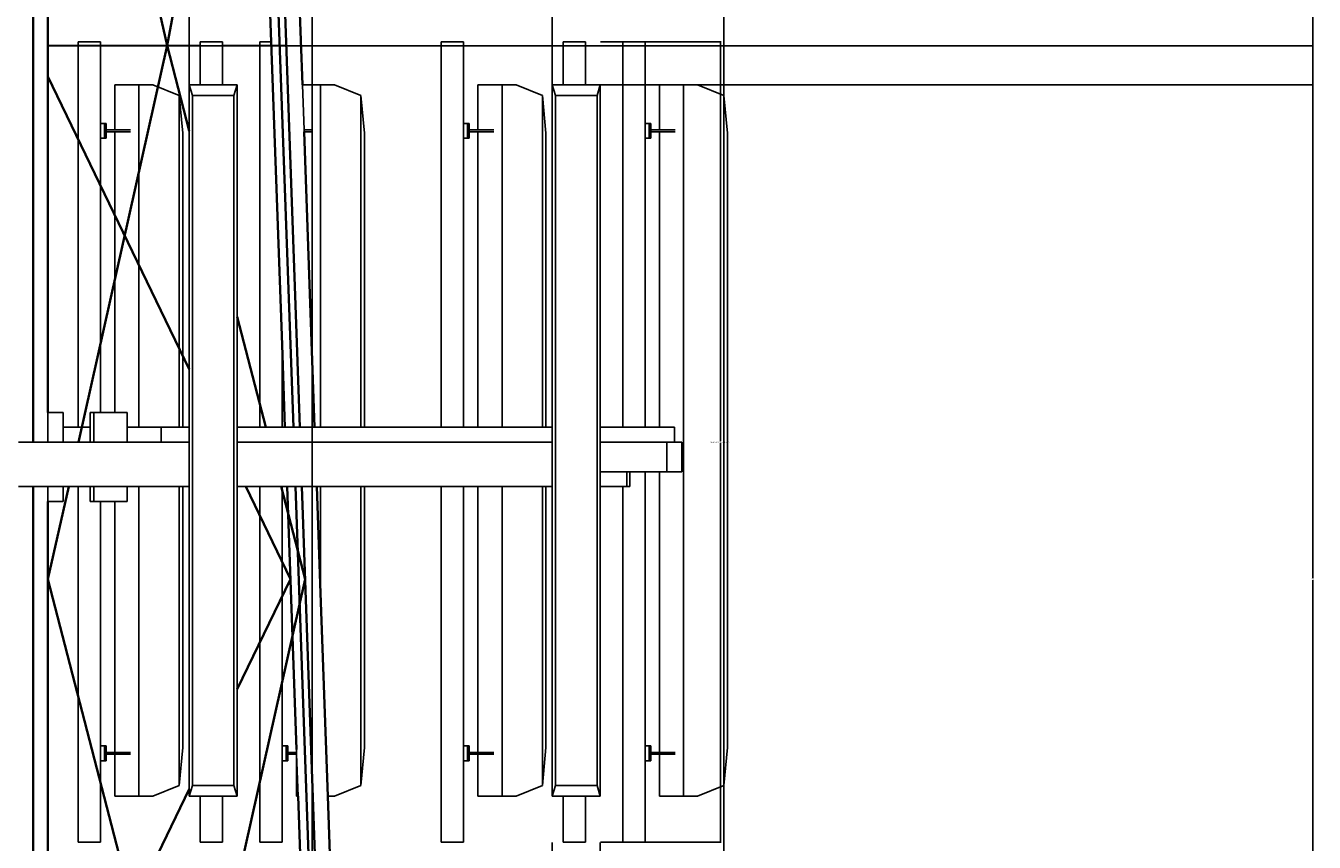
# Model space of a CAD drawing. Units: inches. Extents: x 3780 to 4301, y 1637 to 4224.
# Tile 3 of 8: x 4040 to 4301, y 3092 to 3257. Entities that reach past the tile are written whole.
import ezdxf

# ---------------------------------------------------------------- set-up
doc = ezdxf.new("R2010")
doc.units = ezdxf.units.IN
for name, color, linetype, lineweight in [('A-ANNO-DIMS', 2, 'Continuous', 18), ('E-COMM-ANTN', 4, 'Continuous', 25), ('S-TOWR', 7, 'Continuous', 35)]:
    doc.layers.add(name, color=color, linetype=linetype, lineweight=lineweight)
doc.styles.get("Standard").update_dxf_attribs({"font": 'arial.ttf'})
doc.dimstyles.get("Standard").update_dxf_attribs({"dimtxt": 0.18, "dimasz": 0.18, "dimexe": 0.18, "dimexo": 0.0625, "dimgap": 0.09, "dimtad": 0, "dimtih": 1, "dimtoh": 1, "dimdec": 4, "dimzin": 0, "dimdsep": 46, "dimtxsty": 'Standard', "dimcen": 0.09, "dimadec": 0, "dimazin": 0, "dimtfac": 1, "dimtdec": 4, "dimtofl": 0, "dimtmove": 0, "dimatfit": 3, "dimfxl": 1, "dimtolj": 1, "dimtzin": 0, "dimarcsym": 0})

# ---------------------------------------------------------------- blocks, each defined once
blk = doc.blocks.new('ANT-PANEL')
for p, q in [((3905.38, 3835.91), (3900.05, 3833.75)), ((3905.38, 3835.91), (3908.22, 3835.91)), ((3908.22, 3691.91), (3908.22, 3835.91)), ((3900.05, 3833.75), (3899.34, 3826.07)), ((3900.05, 3694.07), (3900.05, 3833.75)), ((3899.34, 3701.75), (3899.34, 3826.07)), ((3900.05, 3694.07), (3899.34, 3701.75)), ((3905.38, 3691.91), (3900.05, 3694.07)), ((3905.38, 3691.91), (3908.22, 3691.91))]:
    blk.add_line(p, q)
blk = doc.blocks.new('ANT-PANEL-MOUNT-B')
for p, q in [((4148.97, 3835.91), (4148.97, 3844.56)), ((4153.47, 3844.56), (4148.97, 3844.56)), ((4153.47, 3835.91), (4153.47, 3844.56)), ((4146.73, 3835.91), (4147.4, 3833.75)), ((4146.73, 3835.91), (4148.97, 3835.91)), ((4146.73, 3766.56), (4146.73, 3835.91)), ((4148.97, 3835.91), (4153.47, 3835.91)), ((4153.47, 3835.91), (4156.48, 3835.91)), ((4156.48, 3835.91), (4155.82, 3833.75)), ((4156.48, 3766.56), (4156.48, 3835.91)), ((4147.4, 3833.75), (4155.82, 3833.75)), ((4147.4, 3694.07), (4147.4, 3833.75)), ((4155.82, 3694.07), (4155.82, 3833.75)), ((4146.73, 3763.56), (4146.73, 3766.56)), ((4156.48, 3763.56), (4156.48, 3766.56)), ((4146.73, 3754.56), (4146.73, 3763.56)), ((4156.48, 3757.56), (4156.48, 3763.56)), ((4156.48, 3754.56), (4156.48, 3757.56)), ((4146.73, 3691.91), (4146.73, 3754.56)), ((4156.48, 3691.91), (4156.48, 3754.56)), ((4146.73, 3691.91), (4147.4, 3694.07)), ((4147.4, 3694.07), (4155.82, 3694.07)), ((4156.48, 3691.91), (4155.82, 3694.07)), ((4146.73, 3691.91), (4148.97, 3691.91)), ((4148.97, 3682.56), (4148.97, 3691.91)), ((4148.97, 3691.91), (4153.47, 3691.91)), ((4153.47, 3682.56), (4153.47, 3691.91)), ((4153.47, 3691.91), (4156.48, 3691.91)), ((4148.97, 3682.56), (4153.47, 3682.56))]:
    blk.add_line(p, q)
blk = doc.blocks.new('*D9')
at = {"layer": 'A-ANNO-DIMS', "color": 0, "lineweight": -2, "transparency": 16777216}
for p, q in [((4156.54, 3254.21), (4180.96, 3254.21)), ((4180.78, 3254.03), (4180.78, 3173.4)), ((4180.78, 3092.39), (4180.78, 3173.03)), ((4156.54, 3092.21), (4180.96, 3092.21))]:
    blk.add_line(p, q, dxfattribs=at)
at = {"layer": 'A-ANNO-DIMS', "color": 0, "transparency": 16777216}
for points in [[(4180.75, 3254.03), (4180.81, 3254.03), (4180.78, 3254.21)], [(4180.75, 3092.39), (4180.81, 3092.39), (4180.78, 3092.21)]]:
    blk.add_solid(points, dxfattribs=at)
at = {"layer": 'Defpoints', "color": 0, "transparency": 16777216}
for p in [(4156.48, 3254.21), (4180.78, 3254.21), (4156.48, 3092.21)]:
    blk.add_point(p, dxfattribs=at)
at = {"layer": 'A-ANNO-DIMS', "color": 0, "transparency": 16777216, "insert": (4180.78, 3173.21), "char_height": 0.18, "attachment_point": 5}
blk.add_mtext('\\A1;PANEL ANTENNA MOUNT B 162 TYP.', dxfattribs=at)
blk = doc.blocks.new('*D10')
at = {"layer": 'A-ANNO-DIMS', "color": 0, "lineweight": -2, "transparency": 16777216}
for p, q in [((4146.73, 3092.15), (4146.73, 3067.73)), ((4156.48, 3092.15), (4156.48, 3067.73)), ((4146.91, 3067.91), (4151.09, 3067.91)), ((4156.3, 3067.91), (4152.13, 3067.91))]:
    blk.add_line(p, q, dxfattribs=at)
at = {"layer": 'A-ANNO-DIMS', "color": 0, "transparency": 16777216}
for points in [[(4146.91, 3067.94), (4146.91, 3067.88), (4146.73, 3067.91)], [(4156.3, 3067.94), (4156.3, 3067.88), (4156.48, 3067.91)]]:
    blk.add_solid(points, dxfattribs=at)
at = {"layer": 'Defpoints', "color": 0, "transparency": 16777216}
for p in [(4146.73, 3092.21), (4156.48, 3092.21), (4156.48, 3067.91)]:
    blk.add_point(p, dxfattribs=at)
at = {"layer": 'A-ANNO-DIMS', "color": 0, "transparency": 16777216, "insert": (4151.61, 3067.91), "char_height": 0.18, "attachment_point": 5}
blk.add_mtext('\\A1;10 TYP.', dxfattribs=at)
blk = doc.blocks.new('*D19')
at = {"layer": 'A-ANNO-DIMS', "color": 0, "lineweight": -2, "transparency": 16777216}
for p, q in [((4044.72, 3253.46), (4300.89, 3253.46)), ((4300.71, 3253.28), (4300.71, 3145.65)), ((4300.71, 3037.64), (4300.71, 3145.28)), ((4044.72, 3037.46), (4300.89, 3037.46))]:
    blk.add_line(p, q, dxfattribs=at)
at = {"layer": 'A-ANNO-DIMS', "color": 0, "transparency": 16777216}
for points in [[(4300.68, 3253.28), (4300.74, 3253.28), (4300.71, 3253.46)], [(4300.68, 3037.64), (4300.74, 3037.64), (4300.71, 3037.46)]]:
    blk.add_solid(points, dxfattribs=at)
at = {"layer": 'Defpoints', "color": 0, "transparency": 16777216}
for p in [(4044.66, 3253.46), (4300.71, 3253.46), (4044.66, 3037.46)]:
    blk.add_point(p, dxfattribs=at)
at = {"layer": 'A-ANNO-DIMS', "color": 0, "transparency": 16777216, "insert": (4300.71, 3145.46), "char_height": 0.18, "attachment_point": 5}
blk.add_mtext('\\A1;216', dxfattribs=at)
blk = doc.blocks.new('*D20')
at = {"layer": 'A-ANNO-DIMS', "color": 0, "lineweight": -2, "transparency": 16777216}
for p, q in [((4044.72, 3469.46), (4300.89, 3469.46)), ((4300.71, 3469.28), (4300.71, 3361.65)), ((4300.71, 3253.64), (4300.71, 3361.28)), ((4044.72, 3253.46), (4300.89, 3253.46))]:
    blk.add_line(p, q, dxfattribs=at)
at = {"layer": 'A-ANNO-DIMS', "color": 0, "transparency": 16777216}
for points in [[(4300.68, 3469.28), (4300.74, 3469.28), (4300.71, 3469.46)], [(4300.68, 3253.64), (4300.74, 3253.64), (4300.71, 3253.46)]]:
    blk.add_solid(points, dxfattribs=at)
at = {"layer": 'Defpoints', "color": 0, "transparency": 16777216}
for p in [(4044.66, 3469.46), (4300.71, 3469.46), (4044.66, 3253.46)]:
    blk.add_point(p, dxfattribs=at)
at = {"layer": 'A-ANNO-DIMS', "color": 0, "transparency": 16777216, "insert": (4300.71, 3361.46), "char_height": 0.18, "attachment_point": 5}
blk.add_mtext('\\A1;216', dxfattribs=at)
blk = doc.blocks.new('*D22')
at = {"layer": 'A-ANNO-DIMS', "color": 0, "lineweight": -2, "transparency": 16777216}
for p, q in [((3900.05, 3694.01), (3900.05, 1636.57)), ((4181.5, 3694.01), (4181.5, 1636.57)), ((3900.23, 1636.75), (4040.31, 1636.75)), ((4181.32, 1636.75), (4041.24, 1636.75))]:
    blk.add_line(p, q, dxfattribs=at)
at = {"layer": 'A-ANNO-DIMS', "color": 0, "transparency": 16777216}
for points in [[(3900.23, 1636.78), (3900.23, 1636.72), (3900.05, 1636.75)], [(4181.32, 1636.78), (4181.32, 1636.72), (4181.5, 1636.75)]]:
    blk.add_solid(points, dxfattribs=at)
at = {"layer": 'Defpoints', "color": 0, "transparency": 16777216}
for p in [(3900.05, 3694.07), (4181.5, 3694.07), (4181.5, 1636.75)]:
    blk.add_point(p, dxfattribs=at)
at = {"layer": 'A-ANNO-DIMS', "color": 0, "transparency": 16777216, "insert": (4040.77, 1636.75), "char_height": 0.18, "attachment_point": 5}
blk.add_mtext('\\A1;281.45', dxfattribs=at)
blk = doc.blocks.new('*D27')
at = {"layer": 'A-ANNO-DIMS', "color": 0, "lineweight": -2, "transparency": 16777216}
for p, q in [((4048.31, 3488.69), (3780.66, 3488.69)), ((3780.84, 3488.51), (3780.84, 3295.31)), ((3780.84, 3101.74), (3780.84, 3294.94)), ((3926.17, 3101.56), (3780.66, 3101.56))]:
    blk.add_line(p, q, dxfattribs=at)
at = {"layer": 'A-ANNO-DIMS', "color": 0, "transparency": 16777216}
for points in [[(3780.81, 3488.51), (3780.87, 3488.51), (3780.84, 3488.69)], [(3780.81, 3101.74), (3780.87, 3101.74), (3780.84, 3101.56)]]:
    blk.add_solid(points, dxfattribs=at)
at = {"layer": 'Defpoints', "color": 0, "transparency": 16777216}
for p in [(3780.84, 3488.69), (4048.37, 3488.69), (3926.23, 3101.56)]:
    blk.add_point(p, dxfattribs=at)
at = {"layer": 'A-ANNO-DIMS', "color": 0, "transparency": 16777216, "insert": (3780.84, 3295.13), "char_height": 0.18, "attachment_point": 5}
blk.add_mtext('\\A1;387.1', dxfattribs=at)
blk = doc.blocks.new('*D42')
at = {"layer": 'A-ANNO-DIMS', "color": 0, "lineweight": -2, "transparency": 16777216}
for p, q in [((3997.15, 3538.4), (3997.15, 1636.57)), ((4098.15, 3539.64), (4098.15, 1636.57)), ((3997.33, 1636.75), (4047.38, 1636.75)), ((4097.97, 1636.75), (4047.91, 1636.75))]:
    blk.add_line(p, q, dxfattribs=at)
at = {"layer": 'A-ANNO-DIMS', "color": 0, "transparency": 16777216}
for points in [[(3997.33, 1636.78), (3997.33, 1636.72), (3997.15, 1636.75)], [(4097.97, 1636.78), (4097.97, 1636.72), (4098.15, 1636.75)]]:
    blk.add_solid(points, dxfattribs=at)
at = {"layer": 'Defpoints', "color": 0, "transparency": 16777216}
for p in [(3997.15, 3538.47), (4098.15, 3539.7), (4098.15, 1636.75)]:
    blk.add_point(p, dxfattribs=at)
at = {"layer": 'A-ANNO-DIMS', "color": 0, "transparency": 16777216, "insert": (4047.65, 1636.75), "char_height": 0.18, "attachment_point": 5}
blk.add_mtext('\\A1;101', dxfattribs=at)
blk = doc.blocks.new('*D49')
at = {"layer": 'A-ANNO-DIMS', "color": 0, "lineweight": -2, "transparency": 16777216}
for p, q in [((3999.73, 3245.63), (3999.73, 4223.96)), ((3999.91, 4223.78), (4036.16, 4223.78)), ((4073.05, 4223.78), (4036.81, 4223.78)), ((4073.23, 3245.63), (4073.23, 4223.96))]:
    blk.add_line(p, q, dxfattribs=at)
at = {"layer": 'A-ANNO-DIMS', "color": 0, "transparency": 16777216}
for points in [[(3999.91, 4223.81), (3999.91, 4223.75), (3999.73, 4223.78)], [(4073.05, 4223.81), (4073.05, 4223.75), (4073.23, 4223.78)]]:
    blk.add_solid(points, dxfattribs=at)
at = {"layer": 'Defpoints', "color": 0, "transparency": 16777216}
for p in [(4073.23, 4223.78), (3999.73, 3245.56), (4073.23, 3245.56)]:
    blk.add_point(p, dxfattribs=at)
at = {"layer": 'A-ANNO-DIMS', "color": 0, "transparency": 16777216, "insert": (4036.48, 4223.78), "char_height": 0.18, "attachment_point": 5}
blk.add_mtext('\\A1;73.5', dxfattribs=at)
blk = doc.blocks.new('*D50')
at = {"layer": 'A-ANNO-DIMS', "color": 0, "lineweight": -2, "transparency": 16777216}
for p, q in [((4073.23, 3245.63), (4073.23, 4223.96)), ((4073.41, 4223.78), (4109.66, 4223.78)), ((4146.55, 4223.78), (4110.31, 4223.78)), ((4146.73, 3245.63), (4146.73, 4223.96))]:
    blk.add_line(p, q, dxfattribs=at)
at = {"layer": 'A-ANNO-DIMS', "color": 0, "transparency": 16777216}
for points in [[(4073.41, 4223.81), (4073.41, 4223.75), (4073.23, 4223.78)], [(4146.55, 4223.81), (4146.55, 4223.75), (4146.73, 4223.78)]]:
    blk.add_solid(points, dxfattribs=at)
at = {"layer": 'Defpoints', "color": 0, "transparency": 16777216}
for p in [(4146.73, 4223.78), (4073.23, 3245.56), (4146.73, 3245.56)]:
    blk.add_point(p, dxfattribs=at)
at = {"layer": 'A-ANNO-DIMS', "color": 0, "transparency": 16777216, "insert": (4109.98, 4223.78), "char_height": 0.18, "attachment_point": 5}
blk.add_mtext('\\A1;73.5', dxfattribs=at)
blk = doc.blocks.new('*D60')
at = {"layer": 'A-ANNO-DIMS', "color": 0, "lineweight": -2, "transparency": 16777216}
for p, q in [((4170.32, 3280.03), (4300.89, 3280.03)), ((4300.71, 3279.85), (4300.71, 3262.98)), ((4300.71, 3245.74), (4300.71, 3262.62)), ((4156.54, 3245.56), (4300.89, 3245.56))]:
    blk.add_line(p, q, dxfattribs=at)
at = {"layer": 'A-ANNO-DIMS', "color": 0, "transparency": 16777216}
for points in [[(4300.68, 3279.85), (4300.74, 3279.85), (4300.71, 3280.03)], [(4300.68, 3245.74), (4300.74, 3245.74), (4300.71, 3245.56)]]:
    blk.add_solid(points, dxfattribs=at)
at = {"layer": 'Defpoints', "color": 0, "transparency": 16777216}
for p in [(4170.26, 3280.03), (4300.71, 3280.03), (4156.48, 3245.56)]:
    blk.add_point(p, dxfattribs=at)
at = {"layer": 'A-ANNO-DIMS', "color": 0, "transparency": 16777216, "insert": (4300.71, 3262.8), "char_height": 0.18, "attachment_point": 5}
blk.add_mtext('\\A1;34.47', dxfattribs=at)

msp = doc.modelspace()

# ---------------------------------------------------------------- linework, layer by layer
at = {"layer": 'E-COMM-ANTN'}
for p, q in [((4044.6622, 3253.4644), (4068.7741, 3253.4644)), ((4075.4676, 3253.4644), (4044.6622, 3253.4644)), ((4050.7911, 3176.2144), (4050.7911, 3254.2144)), ((4050.7911, 3254.2144), (4055.2911, 3254.2144)), ((4055.2911, 3237.7144), (4055.2911, 3254.2144)), ((4068.7741, 3253.4644), (4075.4676, 3253.4644)), ((4075.4676, 3245.5639), (4075.4676, 3254.2144)), ((4075.4676, 3254.2144), (4079.9676, 3254.2144)), ((4079.9676, 3245.5639), (4079.9676, 3254.2144)), ((4089.886, 3253.4644), (4079.9676, 3253.4644)), ((4079.9676, 3253.4644), (4092.886, 3253.4644)), ((4087.5411, 3176.2144), (4087.5411, 3254.2144)), ((4087.5411, 3254.2144), (4089.8594, 3254.2144)), ((4124.2911, 3176.2144), (4124.2911, 3254.2144)), ((4124.2911, 3254.2144), (4128.7911, 3254.2144)), ((4128.7911, 3237.7144), (4128.7911, 3254.2144)), ((4161.0411, 3176.2144), (4161.0411, 3254.2144)), ((4165.5411, 3254.2144), (4161.0411, 3254.2144)), ((4165.5411, 3237.7144), (4165.5411, 3254.2144)), ((4058.2034, 3236.4019), (4058.2034, 3245.5639)), ((4058.2034, 3245.5639), (4063.0784, 3245.5639)), ((4063.0784, 3245.5639), (4065.9127, 3245.5639)), ((4063.0784, 3176.2144), (4063.0784, 3245.5639)), ((4065.9127, 3245.5639), (4071.248, 3243.4039)), ((4073.2315, 3245.5639), (4073.8979, 3243.4039)), ((4073.2315, 3245.5639), (4075.4676, 3245.5639)), ((4073.2315, 3176.2144), (4073.2315, 3245.5639)), ((4075.4676, 3245.5639), (4079.9676, 3245.5639)), ((4079.9676, 3245.5639), (4082.9815, 3245.5639)), ((4082.9815, 3245.5639), (4082.3151, 3243.4039)), ((4082.9815, 3176.2144), (4082.9815, 3245.5639)), ((4096.4929, 3236.4019), (4096.167, 3245.5639)), ((4096.167, 3245.5639), (4099.8284, 3245.5639)), ((4099.8284, 3176.2144), (4099.8284, 3245.5639)), ((4099.8284, 3245.5639), (4102.6627, 3245.5639)), ((4102.6627, 3245.5639), (4107.998, 3243.4039)), ((4131.7034, 3236.4019), (4131.7034, 3245.5639)), ((4131.7034, 3245.5639), (4136.5784, 3245.5639)), ((4136.5784, 3176.2144), (4136.5784, 3245.5639)), ((4136.5784, 3245.5639), (4139.4127, 3245.5639)), ((4139.4127, 3245.5639), (4144.748, 3243.4039)), ((4168.4534, 3236.4019), (4168.4534, 3245.5639)), ((4168.4534, 3245.5639), (4173.3284, 3245.5639)), ((4071.248, 3176.2144), (4071.248, 3243.4039)), ((4071.248, 3243.4039), (4071.9591, 3235.7215)), ((4073.8979, 3103.7239), (4073.8979, 3243.4039)), ((4073.8979, 3243.4039), (4082.3151, 3243.4039)), ((4082.3151, 3103.7239), (4082.3151, 3243.4039)), ((4107.998, 3243.4039), (4108.7091, 3235.7215)), ((4107.998, 3176.2144), (4107.998, 3243.4039)), ((4144.748, 3243.4039), (4145.4591, 3235.7215)), ((4144.748, 3176.2144), (4144.748, 3243.4039)), ((4055.2911, 3237.7144), (4056.1147, 3237.7144)), ((4055.2911, 3234.7144), (4055.2911, 3237.7144)), ((4056.1147, 3237.7144), (4056.4394, 3237.7144)), ((4056.1147, 3234.7144), (4056.1147, 3237.7144)), ((4056.4394, 3237.7144), (4056.4394, 3236.4019)), ((4128.7911, 3237.7144), (4129.6147, 3237.7144)), ((4128.7911, 3234.7144), (4128.7911, 3237.7144)), ((4129.6147, 3237.7144), (4129.9394, 3237.7144)), ((4129.6147, 3234.7144), (4129.6147, 3237.7144)), ((4129.9394, 3237.7144), (4129.9394, 3236.4019)), ((4165.5411, 3237.7144), (4166.3647, 3237.7144)), ((4165.5411, 3234.7144), (4165.5411, 3237.7144)), ((4166.3647, 3234.7144), (4166.3647, 3237.7144)), ((4166.3647, 3237.7144), (4166.6894, 3237.7144)), ((4166.6894, 3237.7144), (4166.6894, 3236.4019)), ((4055.2911, 3234.7144), (4056.1147, 3234.7144)), ((4055.2911, 3179.2144), (4055.2911, 3234.7144)), ((4056.1147, 3234.7144), (4056.4394, 3234.7144)), ((4058.2034, 3236.4019), (4056.4394, 3236.4019)), ((4056.4394, 3236.4019), (4056.4394, 3236.0269)), ((4056.4394, 3236.0269), (4058.2034, 3236.0269)), ((4056.4394, 3236.0269), (4056.4394, 3234.7144)), ((4058.2034, 3236.4019), (4061.3979, 3236.4019)), ((4058.2034, 3179.2144), (4058.2034, 3236.0269)), ((4058.2034, 3236.0269), (4061.3979, 3236.0269)), ((4071.9591, 3176.2144), (4071.9591, 3235.7215)), ((4096.5062, 3236.0269), (4096.4929, 3236.4019)), ((4096.4929, 3236.4019), (4098.1479, 3236.4019)), ((4096.5062, 3236.0269), (4098.1479, 3236.0269)), ((4108.7091, 3176.2144), (4108.7091, 3235.7215)), ((4128.7911, 3234.7144), (4129.6147, 3234.7144)), ((4128.7911, 3176.2144), (4128.7911, 3234.7144)), ((4129.6147, 3234.7144), (4129.9394, 3234.7144)), ((4131.7034, 3236.4019), (4129.9394, 3236.4019)), ((4129.9394, 3236.4019), (4129.9394, 3236.0269)), ((4129.9394, 3236.0269), (4131.7034, 3236.0269)), ((4129.9394, 3236.0269), (4129.9394, 3234.7144)), ((4131.7034, 3236.4019), (4134.8979, 3236.4019)), ((4131.7034, 3176.2144), (4131.7034, 3236.0269)), ((4131.7034, 3236.0269), (4134.8979, 3236.0269)), ((4145.4591, 3176.2144), (4145.4591, 3235.7215)), ((4165.5411, 3234.7144), (4166.3647, 3234.7144)), ((4165.5411, 3176.2144), (4165.5411, 3234.7144)), ((4166.3647, 3234.7144), (4166.6894, 3234.7144)), ((4166.6894, 3236.4019), (4168.4534, 3236.4019)), ((4166.6894, 3236.4019), (4166.6894, 3236.0269)), ((4166.6894, 3236.0269), (4166.6894, 3234.7144)), ((4166.6894, 3236.0269), (4168.4534, 3236.0269)), ((4168.4534, 3236.4019), (4171.6479, 3236.4019)), ((4168.4534, 3176.2144), (4168.4534, 3236.0269)), ((4168.4534, 3236.0269), (4171.6479, 3236.0269)), ((4092.0411, 3176.2144), (4092.0411, 3192.8708)), ((4047.7176, 3179.2144), (4044.6622, 3179.2144)), ((4044.6622, 3173.2144), (4044.6622, 3179.2144)), ((4047.7176, 3176.2144), (4047.7176, 3179.2144)), ((4053.9472, 3179.2144), (4053.181, 3179.2144)), ((4053.181, 3176.2144), (4053.181, 3179.2144)), ((4053.9472, 3173.2144), (4053.9472, 3179.2144)), ((4053.9472, 3179.2144), (4055.2911, 3179.2144)), ((4055.2911, 3179.2144), (4058.2034, 3179.2144)), ((4060.6972, 3179.2144), (4058.2034, 3179.2144)), ((4060.6972, 3179.2144), (4060.6972, 3176.2144)), ((4047.7176, 3173.2144), (4047.7176, 3176.2144)), ((4047.7176, 3176.2144), (4050.7911, 3176.2144)), ((4050.7911, 3176.2144), (4053.181, 3176.2144)), ((4053.181, 3173.2144), (4053.181, 3176.2144)), ((4060.6972, 3176.2144), (4060.6972, 3173.2144)), ((4060.6972, 3176.2144), (4063.0784, 3176.2144)), ((4063.0784, 3176.2144), (4067.5445, 3176.2144)), ((4067.5445, 3173.2144), (4067.5445, 3176.2144)), ((4071.248, 3176.2144), (4067.5445, 3176.2144)), ((4071.9591, 3176.2144), (4071.248, 3176.2144)), ((4073.2315, 3176.2144), (4071.9591, 3176.2144)), ((4073.2315, 3173.2144), (4073.2315, 3176.2144)), ((4087.5411, 3176.2144), (4082.9815, 3176.2144)), ((4082.9815, 3173.2144), (4082.9815, 3176.2144)), ((4092.0411, 3176.2144), (4087.5411, 3176.2144)), ((4092.6335, 3176.2144), (4092.0411, 3176.2144)), ((4094.3345, 3176.2144), (4092.6335, 3176.2144)), ((4095.6335, 3176.2144), (4094.3345, 3176.2144)), ((4098.6335, 3176.2144), (4095.6335, 3176.2144)), ((4099.8284, 3176.2144), (4098.6335, 3176.2144)), ((4107.998, 3176.2144), (4099.8284, 3176.2144)), ((4108.7091, 3176.2144), (4107.998, 3176.2144)), ((4124.2911, 3176.2144), (4108.7091, 3176.2144)), ((4128.7911, 3176.2144), (4124.2911, 3176.2144)), ((4131.7034, 3176.2144), (4128.7911, 3176.2144)), ((4136.5784, 3176.2144), (4131.7034, 3176.2144)), ((4144.748, 3176.2144), (4136.5784, 3176.2144)), ((4145.4591, 3176.2144), (4144.748, 3176.2144)), ((4146.7315, 3176.2144), (4145.4591, 3176.2144)), ((4161.0411, 3176.2144), (4156.4815, 3176.2144)), ((4165.5411, 3176.2144), (4161.0411, 3176.2144)), ((4168.4534, 3176.2144), (4165.5411, 3176.2144)), ((4171.4676, 3176.2144), (4168.4534, 3176.2144)), ((4171.4676, 3173.2144), (4171.4676, 3176.2144)), ((4041.6622, 3173.2144), (4038.6622, 3173.2144)), ((4044.6622, 3173.2144), (4041.6622, 3173.2144)), ((4047.7176, 3173.2144), (4044.6622, 3173.2144)), ((4053.181, 3173.2144), (4047.7176, 3173.2144)), ((4053.9472, 3173.2144), (4053.181, 3173.2144)), ((4053.9472, 3173.2144), (4060.6972, 3173.2144)), ((4067.5445, 3173.2144), (4060.6972, 3173.2144)), ((4073.2315, 3173.2144), (4067.5445, 3173.2144)), ((4073.2315, 3164.2144), (4073.2315, 3173.2144)), ((4146.7315, 3173.2144), (4082.9815, 3173.2144)), ((4082.9815, 3164.2144), (4082.9815, 3173.2144)), ((4169.976, 3173.2144), (4156.4815, 3173.2144)), ((4169.976, 3167.2144), (4169.976, 3173.2144)), ((4169.976, 3173.2144), (4171.4676, 3173.2144)), ((4172.9591, 3173.2144), (4171.4676, 3173.2144)), ((4172.9591, 3173.2144), (4172.9591, 3167.2144)), ((4161.818, 3167.2144), (4156.4815, 3167.2144)), ((4161.818, 3164.2144), (4161.818, 3167.2144)), ((4162.4676, 3167.2144), (4161.818, 3167.2144)), ((4162.4676, 3164.2144), (4162.4676, 3167.2144)), ((4165.5411, 3167.2144), (4162.4676, 3167.2144)), ((4165.5411, 3111.7144), (4165.5411, 3167.2144)), ((4168.4534, 3167.2144), (4165.5411, 3167.2144)), ((4168.4534, 3110.4019), (4168.4534, 3167.2144)), ((4169.976, 3167.2144), (4168.4534, 3167.2144)), ((4172.9591, 3167.2144), (4169.976, 3167.2144)), ((4038.6622, 3164.2144), (4041.6622, 3164.2144)), ((4041.6622, 3164.2144), (4044.6622, 3164.2144)), ((4044.6622, 3161.2144), (4044.6622, 3164.2144)), ((4044.6622, 3164.2144), (4047.7176, 3164.2144)), ((4047.7176, 3161.2144), (4047.7176, 3164.2144)), ((4047.7176, 3164.2144), (4050.7911, 3164.2144)), ((4050.7911, 3092.2144), (4050.7911, 3164.2144)), ((4050.7911, 3164.2144), (4053.181, 3164.2144)), ((4053.181, 3161.2144), (4053.181, 3164.2144)), ((4053.181, 3164.2144), (4053.9472, 3164.2144)), ((4053.9472, 3161.2144), (4053.9472, 3164.2144)), ((4053.9472, 3164.2144), (4060.6972, 3164.2144)), ((4060.6972, 3164.2144), (4060.6972, 3161.2144)), ((4060.6972, 3164.2144), (4063.0784, 3164.2144)), ((4063.0784, 3101.5639), (4063.0784, 3164.2144)), ((4063.0784, 3164.2144), (4071.248, 3164.2144)), ((4071.248, 3103.7239), (4071.248, 3164.2144)), ((4071.248, 3164.2144), (4071.9591, 3164.2144)), ((4071.9591, 3111.4063), (4071.9591, 3164.2144)), ((4071.9591, 3164.2144), (4073.2315, 3164.2144)), ((4073.2315, 3101.5639), (4073.2315, 3164.2144)), ((4082.9815, 3164.2144), (4087.5411, 3164.2144)), ((4082.9815, 3101.5639), (4082.9815, 3164.2144)), ((4087.5411, 3092.2144), (4087.5411, 3164.2144)), ((4087.5411, 3164.2144), (4092.0411, 3164.2144)), ((4092.0411, 3111.7144), (4092.0411, 3164.2144)), ((4092.0411, 3164.2144), (4093.0603, 3164.2144)), ((4093.0603, 3164.2144), (4094.7613, 3164.2144)), ((4094.7613, 3164.2144), (4096.0603, 3164.2144)), ((4096.0603, 3164.2144), (4099.0603, 3164.2144)), ((4099.0603, 3164.2144), (4099.8284, 3164.2144)), ((4099.8284, 3142.6188), (4099.8284, 3164.2144)), ((4099.8284, 3164.2144), (4107.998, 3164.2144)), ((4107.998, 3103.7239), (4107.998, 3164.2144)), ((4107.998, 3164.2144), (4108.7091, 3164.2144)), ((4108.7091, 3111.4063), (4108.7091, 3164.2144)), ((4108.7091, 3164.2144), (4124.2911, 3164.2144)), ((4124.2911, 3092.2144), (4124.2911, 3164.2144)), ((4124.2911, 3164.2144), (4128.7911, 3164.2144)), ((4128.7911, 3111.7144), (4128.7911, 3164.2144)), ((4128.7911, 3164.2144), (4131.7034, 3164.2144)), ((4131.7034, 3110.4019), (4131.7034, 3164.2144)), ((4131.7034, 3164.2144), (4136.5784, 3164.2144)), ((4136.5784, 3101.5639), (4136.5784, 3164.2144)), ((4136.5784, 3164.2144), (4144.748, 3164.2144)), ((4144.748, 3103.7239), (4144.748, 3164.2144)), ((4144.748, 3164.2144), (4145.4591, 3164.2144)), ((4145.4591, 3111.4063), (4145.4591, 3164.2144)), ((4145.4591, 3164.2144), (4146.7315, 3164.2144)), ((4156.4815, 3164.2144), (4161.0411, 3164.2144)), ((4161.0411, 3092.2144), (4161.0411, 3164.2144)), ((4161.818, 3164.2144), (4161.0411, 3164.2144)), ((4162.4676, 3164.2144), (4161.818, 3164.2144)), ((4044.6622, 3161.2144), (4047.7176, 3161.2144)), ((4053.9472, 3161.2144), (4053.181, 3161.2144)), ((4055.2911, 3161.2144), (4053.9472, 3161.2144)), ((4058.2034, 3161.2144), (4055.2911, 3161.2144)), ((4055.2911, 3111.7144), (4055.2911, 3161.2144)), ((4058.2034, 3110.4019), (4058.2034, 3161.2144)), ((4060.6972, 3161.2144), (4058.2034, 3161.2144)), ((4055.2911, 3111.7144), (4056.1147, 3111.7144)), ((4055.2911, 3108.7144), (4055.2911, 3111.7144)), ((4056.1147, 3111.7144), (4056.4394, 3111.7144)), ((4056.1147, 3108.7144), (4056.1147, 3111.7144)), ((4056.4394, 3111.7144), (4056.4394, 3110.4019)), ((4058.2034, 3110.4019), (4056.4394, 3110.4019)), ((4056.4394, 3110.4019), (4056.4394, 3110.0269)), ((4056.4394, 3110.0269), (4058.2034, 3110.0269)), ((4056.4394, 3110.0269), (4056.4394, 3108.7144)), ((4058.2034, 3110.4019), (4061.3979, 3110.4019)), ((4058.2034, 3101.5639), (4058.2034, 3110.0269)), ((4058.2034, 3110.0269), (4061.3979, 3110.0269)), ((4071.248, 3103.7239), (4071.9591, 3111.4063)), ((4092.0411, 3111.7144), (4092.8647, 3111.7144)), ((4092.0411, 3108.7144), (4092.0411, 3111.7144)), ((4092.8647, 3108.7144), (4092.8647, 3111.7144)), ((4092.8647, 3111.7144), (4093.1894, 3111.7144)), ((4093.1894, 3111.7144), (4093.1894, 3110.4019)), ((4094.9534, 3110.4019), (4093.1894, 3110.4019)), ((4093.1894, 3110.4019), (4093.1894, 3110.0269)), ((4093.1894, 3110.0269), (4093.1894, 3108.7144)), ((4093.1894, 3110.0269), (4094.9534, 3110.0269)), ((4094.9534, 3110.4019), (4094.9534, 3110.9877)), ((4094.9742, 3110.4019), (4094.9534, 3110.9877)), ((4094.9742, 3110.4019), (4094.9534, 3110.4019)), ((4094.9534, 3101.5639), (4094.9534, 3110.0269)), ((4094.9534, 3110.0269), (4094.9876, 3110.0269)), ((4094.9876, 3110.0269), (4094.9742, 3110.4019)), ((4095.2886, 3101.5639), (4094.9876, 3110.0269)), ((4107.998, 3103.7239), (4108.7091, 3111.4063)), ((4128.7911, 3111.7144), (4129.6147, 3111.7144)), ((4128.7911, 3108.7144), (4128.7911, 3111.7144)), ((4129.6147, 3111.7144), (4129.9394, 3111.7144)), ((4129.6147, 3108.7144), (4129.6147, 3111.7144)), ((4129.9394, 3111.7144), (4129.9394, 3110.4019)), ((4131.7034, 3110.4019), (4129.9394, 3110.4019)), ((4129.9394, 3110.4019), (4129.9394, 3110.0269)), ((4129.9394, 3110.0269), (4129.9394, 3108.7144)), ((4129.9394, 3110.0269), (4131.7034, 3110.0269)), ((4131.7034, 3110.4019), (4134.8979, 3110.4019)), ((4131.7034, 3101.5639), (4131.7034, 3110.0269)), ((4131.7034, 3110.0269), (4134.8979, 3110.0269)), ((4144.748, 3103.7239), (4145.4591, 3111.4063)), ((4165.5411, 3111.7144), (4166.3647, 3111.7144)), ((4165.5411, 3108.7144), (4165.5411, 3111.7144)), ((4166.3647, 3111.7144), (4166.6894, 3111.7144)), ((4166.3647, 3108.7144), (4166.3647, 3111.7144)), ((4166.6894, 3111.7144), (4166.6894, 3110.4019)), ((4168.4534, 3110.4019), (4166.6894, 3110.4019)), ((4166.6894, 3110.4019), (4166.6894, 3110.0269)), ((4166.6894, 3110.0269), (4168.4534, 3110.0269)), ((4166.6894, 3110.0269), (4166.6894, 3108.7144)), ((4168.4534, 3110.4019), (4171.6479, 3110.4019)), ((4168.4534, 3101.5639), (4168.4534, 3110.0269)), ((4168.4534, 3110.0269), (4171.6479, 3110.0269)), ((4055.2911, 3108.7144), (4056.1147, 3108.7144)), ((4055.2911, 3092.2144), (4055.2911, 3108.7144)), ((4056.1147, 3108.7144), (4056.4394, 3108.7144)), ((4092.0411, 3108.7144), (4092.8647, 3108.7144)), ((4092.0411, 3092.2144), (4092.0411, 3108.7144)), ((4092.8647, 3108.7144), (4093.1894, 3108.7144)), ((4128.7911, 3108.7144), (4129.6147, 3108.7144)), ((4128.7911, 3092.2144), (4128.7911, 3108.7144)), ((4129.6147, 3108.7144), (4129.9394, 3108.7144)), ((4165.5411, 3108.7144), (4166.3647, 3108.7144)), ((4165.5411, 3092.2144), (4165.5411, 3108.7144)), ((4166.3647, 3108.7144), (4166.6894, 3108.7144)), ((4063.0784, 3101.5639), (4058.2034, 3101.5639)), ((4063.0784, 3101.5639), (4065.9127, 3101.5639)), ((4065.9127, 3101.5639), (4071.248, 3103.7239)), ((4073.2315, 3101.5639), (4073.8979, 3103.7239)), ((4073.2315, 3101.5639), (4075.4676, 3101.5639)), ((4073.8979, 3103.7239), (4082.3151, 3103.7239)), ((4075.4676, 3092.2144), (4075.4676, 3101.5639)), ((4075.4676, 3101.5639), (4079.9676, 3101.5639)), ((4079.9676, 3092.2144), (4079.9676, 3101.5639)), ((4079.9676, 3101.5639), (4082.9815, 3101.5639)), ((4082.9815, 3101.5639), (4082.3151, 3103.7239)), ((4095.2886, 3101.5639), (4094.9534, 3101.5639)), ((4101.2886, 3101.5639), (4102.6627, 3101.5639)), ((4102.6627, 3101.5639), (4107.998, 3103.7239)), ((4136.5784, 3101.5639), (4131.7034, 3101.5639)), ((4136.5784, 3101.5639), (4139.4127, 3101.5639)), ((4139.4127, 3101.5639), (4144.748, 3103.7239)), ((4173.3284, 3101.5639), (4168.4534, 3101.5639)), ((4055.2911, 3092.2144), (4050.7911, 3092.2144)), ((4075.4676, 3092.2144), (4079.9676, 3092.2144)), ((4087.5411, 3092.2144), (4092.0411, 3092.2144)), ((4124.2911, 3092.2144), (4128.7911, 3092.2144)), ((4161.0411, 3092.2144), (4165.5411, 3092.2144))]:
    msp.add_line(p, q, dxfattribs=at)
at = {"layer": 'S-TOWR'}
for p, q in [((4041.6622, 3173.2144), (4041.6622, 3489.463)), ((4044.6622, 3179.2144), (4044.6622, 3489.1052)), ((4089.8594, 3254.2144), (4081.6516, 3484.9897)), ((4068.7741, 3253.4644), (4044.6622, 3361.4644)), ((4088.1565, 3356.7311), (4068.7741, 3253.4644)), ((4094.3345, 3176.2144), (4089.8251, 3303.0018)), ((4091.125, 3302.978), (4095.6335, 3176.2144)), ((4096.167, 3245.5639), (4094.127, 3302.9229)), ((4050.8576, 3173.2144), (4068.7741, 3253.4644)), ((4068.7741, 3253.4644), (4073.2315, 3236.2429)), ((4092.0411, 3192.8708), (4089.8594, 3254.2144)), ((4073.2315, 3187.9793), (4044.6622, 3247.2414)), ((4098.6335, 3176.2144), (4096.5062, 3236.0269)), ((4082.9815, 3198.5726), (4088.7683, 3176.2144)), ((4092.6335, 3176.2144), (4092.0411, 3192.8708)), ((4041.6622, 1755.2487), (4041.6622, 3164.2144)), ((4044.6622, 3145.4644), (4048.8483, 3164.2144)), ((4093.7272, 3145.4644), (4084.6881, 3164.2144)), ((4091.8742, 3164.2144), (4096.7272, 3145.4644)), ((4094.9534, 3110.9877), (4093.0603, 3164.2144)), ((4144.8729, 1755.2487), (4094.7613, 3164.2144)), ((4146.1719, 1755.2487), (4096.0603, 3164.2144)), ((4099.8284, 3142.6188), (4099.0603, 3164.2144)), ((4044.6622, 1755.2487), (4044.6622, 3161.2144)), ((4072.6153, 3037.4644), (4044.6622, 3145.4644)), ((4096.7272, 3145.4644), (4072.6153, 3037.4644)), ((4082.9815, 3123.1743), (4093.7272, 3145.4644)), ((4101.2886, 3101.5639), (4099.8284, 3142.6188)), ((4044.6622, 3043.6874), (4073.2315, 3102.9495)), ((4143.1719, 1755.2487), (4095.2886, 3101.5639)), ((4149.1719, 1755.2487), (4101.2886, 3101.5639))]:
    msp.add_line(p, q, dxfattribs=at)

# ---------------------------------------------------------------- block references
at = {"layer": 'E-COMM-ANTN'}
msp.add_blockref('ANT-PANEL-MOUNT-B', (0, -590.3437), dxfattribs=at)
at = {"layer": 'E-COMM-ANTN', "rotation": 180}
msp.add_blockref('ANT-PANEL', (8081.5462, 6937.4716), dxfattribs=at)

# ---------------------------------------------------------------- dimensions: what is measured, and where the dimension line sits
at = {"layer": 'A-ANNO-DIMS'}
for base, p1, p2, override, picture, middle in [((4073.2315, 4223.7769), (3999.7315, 3245.5639), (4073.2315, 3245.5639), {"dimdec": 1, "dimlfac": 1, "dimrnd": 0, "dimzin": 0, "dimdsep": 46, "dimlunit": 2}, '*D49', (4036.4815, 4223.7769)), ((4146.7315, 4223.7769), (4073.2315, 3245.5639), (4146.7315, 3245.5639), {"dimdec": 1, "dimlfac": 1, "dimrnd": 0, "dimzin": 0, "dimdsep": 46, "dimlunit": 2}, '*D50', (4109.9815, 4223.7769)), ((4181.498, 1636.7487), (3900.0482, 3694.0677), (4181.498, 3694.0677), {"dimdec": 2, "dimlfac": 1, "dimrnd": 0, "dimzin": 0, "dimdsep": 46, "dimlunit": 2}, '*D22', (4040.7731, 1636.7487)), ((4098.1498, 1636.7487), (3997.1451, 3538.4672), (4098.1498, 3539.6986), {"dimdec": 0, "dimlfac": 1, "dimrnd": 0, "dimzin": 0, "dimdsep": 46, "dimlunit": 2}, '*D42', (4047.6474, 1636.7487))]:
    dim = msp.add_linear_dim(base=base, p1=p1, p2=p2, dimstyle='Standard', override=override, dxfattribs=at)
    dim.commit()
    dim.dimension.update_dxf_attribs({"geometry": picture, "text_midpoint": middle})
for base, p1, p2, override, picture, middle in [((3780.8371, 3488.689), (3926.2315, 3101.5639), (4048.3735, 3488.689), {"dimdec": 1, "dimlfac": 1, "dimrnd": 0, "dimzin": 0, "dimdsep": 46, "dimlunit": 2}, '*D27', (3780.8371, 3295.1265)), ((4300.7091, 3469.4644), (4044.6622, 3253.4644), (4044.6622, 3469.4644), {"dimdec": 0, "dimlfac": 1, "dimrnd": 0, "dimzin": 0, "dimdsep": 46, "dimlunit": 2}, '*D20', (4300.7091, 3361.4644)), ((4300.7091, 3280.034), (4156.4815, 3245.5639), (4170.2605, 3280.034), {"dimdec": 2, "dimlfac": 1, "dimrnd": 0, "dimzin": 0, "dimdsep": 46, "dimlunit": 2}, '*D60', (4300.7091, 3262.799)), ((4300.7091, 3253.4644), (4044.6622, 3037.4644), (4044.6622, 3253.4644), {"dimdec": 0, "dimlfac": 1, "dimrnd": 0, "dimzin": 0, "dimdsep": 46, "dimlunit": 2}, '*D19', (4300.7091, 3145.4644))]:
    dim = msp.add_linear_dim(base=base, p1=p1, p2=p2, angle=90, dimstyle='Standard', override=override, dxfattribs=at)
    dim.commit()
    dim.dimension.update_dxf_attribs({"geometry": picture, "text_midpoint": middle})
dim = msp.add_linear_dim(base=(4180.7815, 3254.2144), p1=(4156.4815, 3092.2144), p2=(4156.4815, 3254.2144), angle=90, text='PANEL ANTENNA MOUNT B <> TYP.', dimstyle='Standard', override={"dimdec": 0, "dimlfac": 1, "dimrnd": 0, "dimzin": 0, "dimdsep": 46, "dimlunit": 2}, dxfattribs=at)
dim.commit()
dim.dimension.update_dxf_attribs({"geometry": '*D9', "text_midpoint": (4180.7815, 3173.2144)})
dim = msp.add_linear_dim(base=(4156.4815, 3067.9144), p1=(4146.7315, 3092.2144), p2=(4156.4815, 3092.2144), text='<> TYP.', dimstyle='Standard', override={"dimdec": 0, "dimlfac": 1, "dimrnd": 0, "dimzin": 0, "dimdsep": 46, "dimlunit": 2}, dxfattribs=at)
dim.commit()
dim.dimension.update_dxf_attribs({"geometry": '*D10', "text_midpoint": (4151.6065, 3067.9144)})

doc.saveas('drawing.dxf')
